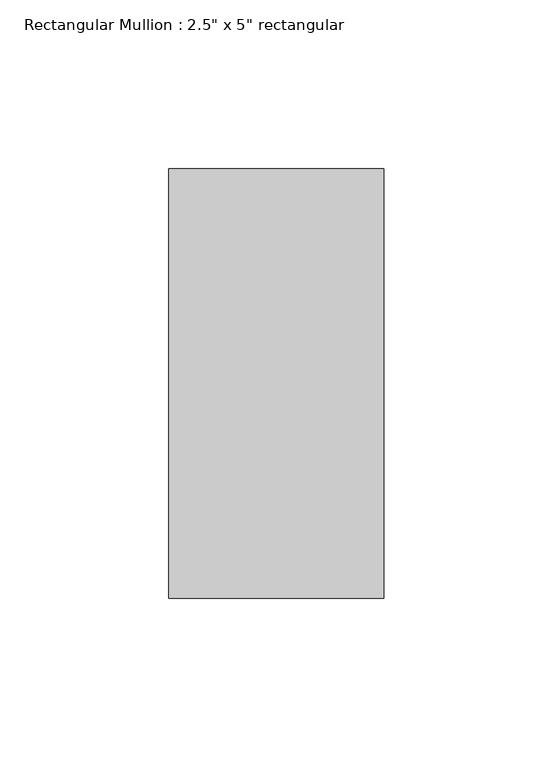
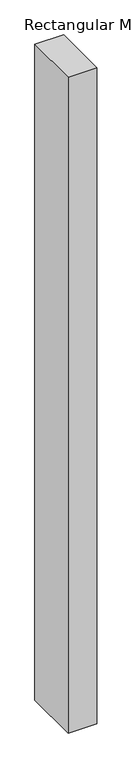
"""IFC4 building model written with IfcOpenShell, lengths in millimetres: member geometry."""

from ifc_helpers import new_model, si_unit, frame, origin, place, context, project, spatial, polyline, outline, extrude, source, transform, mapped, element, save


def member_a8b9c919(model_context):
    return source(origin(), model_context, "Body", "SweptSolid", [
        extrude(outline(polyline([(31.75, 63.5), (31.75, -63.5), (-31.75, -63.5), (-31.75, 63.5), (31.75, 63.5)])), frame((0.0, 0.0, -1536.2264761), z_axis=(0.0, 0.0, 1.0), x_axis=(1.0, 0.0, 0.0)), (0.0, 0.0, 1.0), 1536.2264761),
    ])


if __name__ == "__main__":
    model = new_model("IFC4")
    model_context = context("Model", 3, world=origin())
    ifc_project = project(units=[si_unit("LENGTHUNIT", "METRE", prefix="MILLI")], contexts=[model_context])
    site = spatial("IfcSite", under=ifc_project)
    building = spatial("IfcBuilding", under=site)
    placement = place(None, origin())
    member_shape = member_a8b9c919(model_context)
    element("IfcMember", 1, ObjectType="Rectangular Mullion : 2.5\" x 5\" rectangular", at=placement, inside=building, context=model_context, shape_type="MappedRepresentation", body=[
        mapped(member_shape, transform((0.0, 0.0, 0.0), x_axis=(1.0, 0.0, 0.0), y_axis=(0.0, 1.0, 0.0), z_axis=(0.0, 0.0, 1.0))),
    ])
    save(model, "model.ifc")

# Revit data of these elements
# Type "Rectangular Mullion : 2.5\" x 5\" rectangular"
#   built-in parameter 1007304 = 0.416667 (stored number, unit not read)
#   built-in parameter 1007301 = 0.104167 (stored number, unit not read)
#   built-in parameter 1007300 = 0.104167 (stored number, unit not read)
# Element 1 (IfcMember, "Rectangular Mullion : 2.5\" x 5\" rectangular")
#   Materials on its faces: "Aluminum"
# Materials
#   "Aluminum": class "Metal", colour RGB 247 247 247, transparency 0, Description = "Aluminum 6061", Cost = 0
